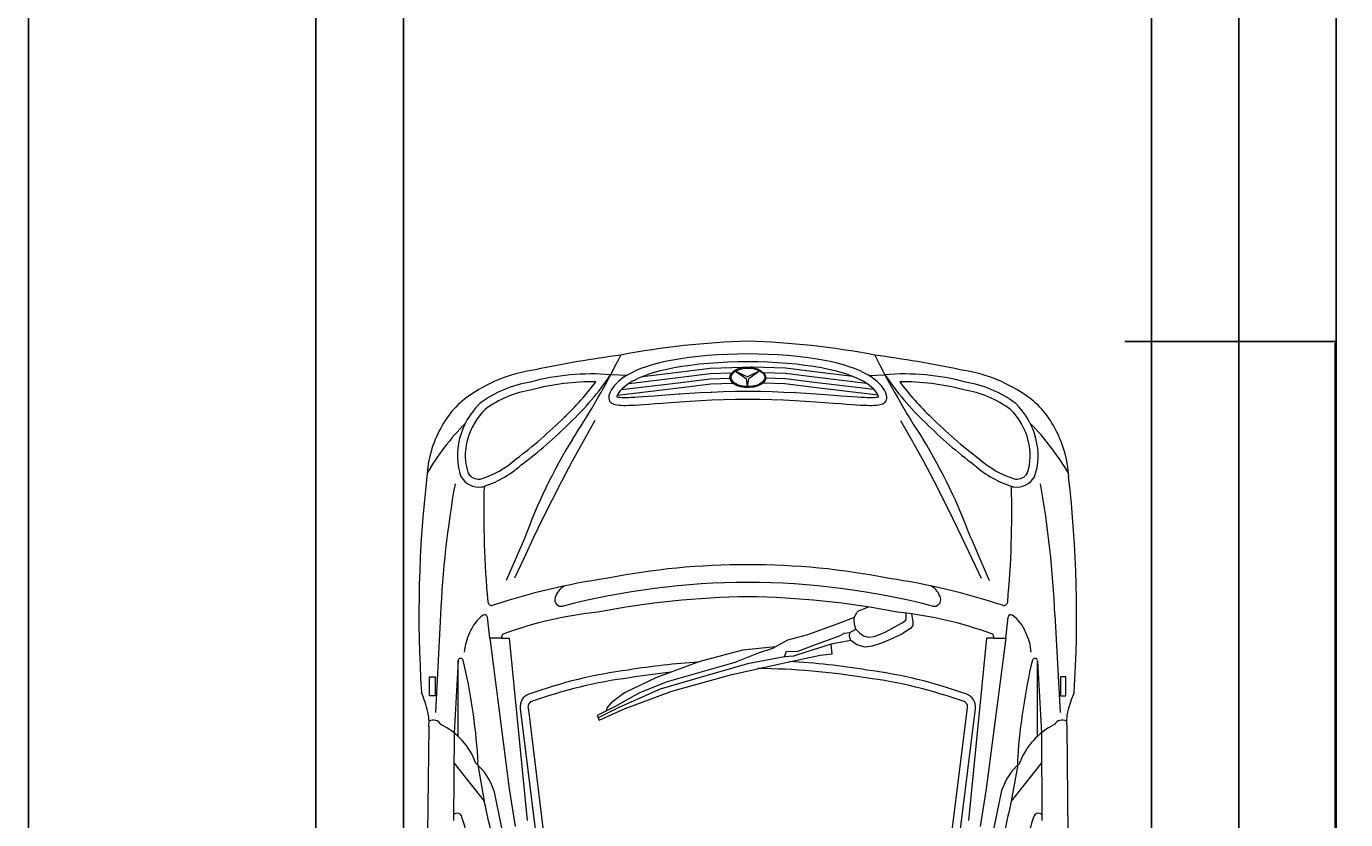
# Model space of a CAD drawing. Units: inches. Extents: x 450 to 1026, y 542 to 1190.
# Tile 3 of 11: x 450 to 586, y 723 to 804. Entities that reach past the tile are written whole.
import ezdxf

# ---------------------------------------------------------------- set-up
doc = ezdxf.new("R2010")
doc.units = ezdxf.units.IN
doc.header["$MEASUREMENT"] = 0
for name, color, linetype, lineweight in [('A-ANNO-DIMS', 2, 'Continuous', 18), ('A-FLOR', 8, 'Continuous', 25), ('C-PROP', 7, 'Continuous', 25), ('C-SITE-VEHC', 8, 'Continuous', 13)]:
    doc.layers.add(name, color=color, linetype=linetype, lineweight=lineweight)
doc.styles.get("Standard").update_dxf_attribs({"font": 'arial.ttf'})
doc.dimstyles.get("Standard").update_dxf_attribs({"dimtxt": 0.18, "dimasz": 0.18, "dimexe": 0.18, "dimexo": 0.0625, "dimgap": 0.09, "dimtad": 0, "dimtih": 1, "dimtoh": 1, "dimdec": 4, "dimzin": 0, "dimdsep": 46, "dimtxsty": 'Standard', "dimcen": 0.09, "dimadec": 0, "dimazin": 0, "dimtfac": 1, "dimtdec": 4, "dimtofl": 0, "dimtmove": 0, "dimatfit": 3, "dimfxl": 1, "dimtolj": 1, "dimtzin": 0, "dimarcsym": 0})

# ---------------------------------------------------------------- blocks, each defined once
blk = doc.blocks.new('A$C27D64469')
for p, q in [((-0.0377, -0.4341), (-0.0629, -0.4354)), ((-0.0122, -0.4333), (-0.0377, -0.4341)), ((0.0136, -0.433), (-0.0122, -0.4333)), ((0.0393, -0.4333), (0.0136, -0.433)), ((0.0649, -0.4341), (0.0393, -0.4333)), ((0.0901, -0.4354), (0.0649, -0.4341)), ((-0.2436, -0.4655), (-0.2571, -0.4703)), ((-0.2289, -0.4609), (-0.2436, -0.4655)), ((-0.2128, -0.4566), (-0.2289, -0.4609)), ((-0.1954, -0.4525), (-0.2128, -0.4566)), ((-0.1764, -0.4487), (-0.1954, -0.4525)), ((-0.156, -0.4453), (-0.1764, -0.4487)), ((-0.153, -0.4651), (-0.1728, -0.4684)), ((-0.1343, -0.4422), (-0.156, -0.4453)), ((-0.1317, -0.4621), (-0.153, -0.4651)), ((-0.1114, -0.4395), (-0.1343, -0.4422)), ((-0.1093, -0.4594), (-0.1317, -0.4621)), ((-0.0875, -0.4373), (-0.1114, -0.4395)), ((-0.0858, -0.4572), (-0.1093, -0.4594)), ((-0.0629, -0.4354), (-0.0875, -0.4373)), ((-0.0616, -0.4554), (-0.0858, -0.4572)), ((-0.0819, -0.4693), (0.0012, -0.4665)), ((-0.0369, -0.4541), (-0.0616, -0.4554)), ((-0.0117, -0.4533), (-0.0369, -0.4541)), ((0.0136, -0.453), (-0.0117, -0.4533)), ((0.0012, -0.4665), (0.0067, -0.4665)), ((0.0389, -0.4533), (0.0136, -0.453)), ((0.0259, -0.4665), (0.0204, -0.4665)), ((0.109, -0.4693), (0.0259, -0.4665)), ((0.064, -0.4541), (0.0389, -0.4533)), ((0.0888, -0.4554), (0.064, -0.4541)), ((0.113, -0.4572), (0.0888, -0.4554)), ((0.1147, -0.4373), (0.0901, -0.4354)), ((0.1364, -0.4594), (0.113, -0.4572)), ((0.1385, -0.4395), (0.1147, -0.4373)), ((0.1588, -0.4621), (0.1364, -0.4594)), ((0.1614, -0.4422), (0.1385, -0.4395)), ((0.1801, -0.4651), (0.1588, -0.4621)), ((0.1832, -0.4453), (0.1614, -0.4422)), ((0.2, -0.4684), (0.1801, -0.4651)), ((0.2036, -0.4487), (0.1832, -0.4453)), ((0.2225, -0.4525), (0.2036, -0.4487)), ((0.24, -0.4566), (0.2225, -0.4525)), ((0.2561, -0.4609), (0.24, -0.4566)), ((0.2708, -0.4655), (0.2561, -0.4609)), ((0.2842, -0.4703), (0.2708, -0.4655)), ((-0.2923, -0.4873), (-0.3337, -0.4857)), ((-0.307, -0.4972), (-0.3138, -0.5028)), ((-0.2991, -0.4915), (-0.307, -0.4972)), ((-0.2902, -0.486), (-0.2991, -0.4915)), ((-0.2803, -0.4806), (-0.2902, -0.486)), ((-0.287, -0.5076), (-0.1557, -0.4919)), ((-0.2693, -0.4753), (-0.2803, -0.4806)), ((-0.2712, -0.4984), (-0.2801, -0.5033)), ((-0.2612, -0.4936), (-0.2712, -0.4984)), ((-0.2571, -0.4703), (-0.2693, -0.4753)), ((-0.2499, -0.489), (-0.2612, -0.4936)), ((-0.253, -0.4902), (-0.1557, -0.4786)), ((-0.2373, -0.4844), (-0.2499, -0.489)), ((-0.2233, -0.4801), (-0.2373, -0.4844)), ((-0.208, -0.476), (-0.2233, -0.4801)), ((-0.1912, -0.4721), (-0.208, -0.476)), ((-0.1728, -0.4684), (-0.1912, -0.4721)), ((-0.1557, -0.4786), (-0.0819, -0.4693)), ((-0.1557, -0.4919), (-0.0819, -0.4825)), ((-0.1557, -0.5051), (-0.0819, -0.4958)), ((-0.0819, -0.4825), (-0.0265, -0.4807)), ((-0.0819, -0.4958), (-0.0315, -0.4941)), ((-0.0174, -0.4766), (0.0132, -0.4908)), ((-0.0174, -0.4766), (0.0101, -0.4961)), ((0.0133, -0.5159), (0.0101, -0.4961)), ((0.0445, -0.4762), (0.0132, -0.4908)), ((0.0133, -0.5159), (0.0162, -0.4961)), ((0.0445, -0.4762), (0.0162, -0.4961)), ((0.109, -0.4825), (0.0537, -0.4807)), ((0.109, -0.4958), (0.0586, -0.4941)), ((0.1828, -0.4786), (0.109, -0.4693)), ((0.1828, -0.4919), (0.109, -0.4825)), ((0.1828, -0.5051), (0.109, -0.4958)), ((0.2801, -0.4902), (0.1828, -0.4786)), ((0.3141, -0.5076), (0.1828, -0.4919)), ((0.2183, -0.4721), (0.2, -0.4684)), ((0.2351, -0.476), (0.2183, -0.4721)), ((0.2505, -0.4801), (0.2351, -0.476)), ((0.2644, -0.4844), (0.2505, -0.4801)), ((0.277, -0.489), (0.2644, -0.4844)), ((0.2883, -0.4936), (0.277, -0.489)), ((0.2964, -0.4753), (0.2842, -0.4703)), ((0.2984, -0.4984), (0.2883, -0.4936)), ((0.3075, -0.4806), (0.2964, -0.4753)), ((0.3073, -0.5033), (0.2984, -0.4984)), ((0.3174, -0.486), (0.3075, -0.4806)), ((0.3262, -0.4915), (0.3174, -0.486)), ((0.3195, -0.4873), (0.3609, -0.4857)), ((0.3341, -0.4972), (0.3262, -0.4915)), ((0.341, -0.5028), (0.3341, -0.4972)), ((-0.3369, -0.5343), (-0.3381, -0.5386)), ((-0.3351, -0.5296), (-0.3369, -0.5343)), ((-0.3324, -0.5247), (-0.3351, -0.5296)), ((-0.329, -0.5195), (-0.3324, -0.5247)), ((-0.3248, -0.514), (-0.329, -0.5195)), ((-0.3198, -0.5085), (-0.3248, -0.514)), ((-0.3138, -0.5028), (-0.3198, -0.5085)), ((-0.3166, -0.5376), (-0.154, -0.5181)), ((-0.3127, -0.5311), (-0.3152, -0.5348)), ((-0.3095, -0.5269), (-0.3127, -0.5311)), ((-0.3055, -0.5225), (-0.3095, -0.5269)), ((-0.306, -0.5231), (-0.1557, -0.5051)), ((-0.3006, -0.5178), (-0.3055, -0.5225)), ((-0.2947, -0.513), (-0.3006, -0.5178)), ((-0.288, -0.5082), (-0.2947, -0.513)), ((-0.2883, -0.5077), (-0.2883, -0.5077)), ((-0.2801, -0.5033), (-0.288, -0.5082)), ((-0.1832, -0.5361), (-0.1598, -0.5344)), ((-0.1597, -0.5344), (-0.1342, -0.5327)), ((-0.154, -0.5181), (-0.0802, -0.5088)), ((-0.1341, -0.5327), (-0.1069, -0.5311)), ((-0.1067, -0.5311), (-0.0781, -0.5297)), ((-0.0802, -0.5088), (-0.0242, -0.5069)), ((-0.0779, -0.5297), (-0.0482, -0.5285)), ((-0.048, -0.5285), (-0.0176, -0.5278)), ((-0.0173, -0.5278), (0.0134, -0.5275)), ((0.0138, -0.5275), (0.0444, -0.5278)), ((0.0448, -0.5278), (0.0751, -0.5285)), ((0.1074, -0.5088), (0.0513, -0.5069)), ((0.0754, -0.5285), (0.105, -0.5297)), ((0.1052, -0.5297), (0.1339, -0.5311)), ((0.1811, -0.5181), (0.1074, -0.5088)), ((0.134, -0.5311), (0.1612, -0.5327)), ((0.1614, -0.5327), (0.1869, -0.5344)), ((0.3438, -0.5376), (0.1811, -0.5181)), ((0.3332, -0.5231), (0.1828, -0.5051)), ((0.187, -0.5344), (0.2103, -0.5361)), ((0.3151, -0.5082), (0.3073, -0.5033)), ((0.3219, -0.513), (0.3151, -0.5082)), ((0.3277, -0.5178), (0.3219, -0.513)), ((0.3326, -0.5225), (0.3277, -0.5178)), ((0.3367, -0.5269), (0.3326, -0.5225)), ((0.3399, -0.5311), (0.3367, -0.5269)), ((0.3423, -0.5348), (0.3399, -0.5311)), ((0.3469, -0.5085), (0.341, -0.5028)), ((0.352, -0.514), (0.3469, -0.5085)), ((0.3562, -0.5195), (0.352, -0.514)), ((0.3596, -0.5247), (0.3562, -0.5195)), ((0.3622, -0.5296), (0.3596, -0.5247)), ((0.3641, -0.5343), (0.3622, -0.5296)), ((0.3653, -0.5386), (0.3641, -0.5343)), ((-0.3381, -0.5386), (-0.3386, -0.5425)), ((-0.3386, -0.5425), (-0.3385, -0.5462)), ((-0.3385, -0.5462), (-0.3378, -0.5495)), ((-0.3378, -0.5495), (-0.3364, -0.5524)), ((-0.3364, -0.5524), (-0.3345, -0.5549)), ((-0.3345, -0.5549), (-0.3321, -0.5571)), ((-0.3321, -0.5571), (-0.3292, -0.5589)), ((-0.3292, -0.5589), (-0.3258, -0.5604)), ((-0.3258, -0.5604), (-0.3219, -0.5615)), ((-0.3219, -0.5615), (-0.3175, -0.5623)), ((-0.318, -0.5407), (-0.3183, -0.5417)), ((-0.3183, -0.5417), (-0.3172, -0.542)), ((-0.3169, -0.5381), (-0.318, -0.5407)), ((-0.3175, -0.5623), (-0.3126, -0.5629)), ((-0.3172, -0.542), (-0.3144, -0.5426)), ((-0.3152, -0.5348), (-0.3169, -0.5381)), ((-0.3144, -0.5426), (-0.3108, -0.543)), ((-0.3126, -0.5629), (-0.3072, -0.5633)), ((-0.3108, -0.543), (-0.3063, -0.5433)), ((-0.3072, -0.5633), (-0.3014, -0.5634)), ((-0.3063, -0.5433), (-0.3012, -0.5434)), ((-0.3014, -0.5634), (-0.2951, -0.5634)), ((-0.3012, -0.5434), (-0.2953, -0.5434)), ((-0.2953, -0.5434), (-0.2888, -0.5433)), ((-0.2951, -0.5634), (-0.2882, -0.5633)), ((-0.2888, -0.5433), (-0.2815, -0.543)), ((-0.2882, -0.5633), (-0.2806, -0.563)), ((-0.2815, -0.543), (-0.2731, -0.5425)), ((-0.2806, -0.563), (-0.272, -0.5625)), ((-0.2731, -0.5425), (-0.2632, -0.5419)), ((-0.272, -0.5625), (-0.2619, -0.5619)), ((-0.2632, -0.5419), (-0.2517, -0.5411)), ((-0.2619, -0.5619), (-0.2503, -0.5611)), ((-0.2517, -0.5411), (-0.2382, -0.5402)), ((-0.2503, -0.5611), (-0.2367, -0.5601)), ((-0.2382, -0.5402), (-0.2225, -0.539)), ((-0.2367, -0.5601), (-0.221, -0.559)), ((-0.2225, -0.539), (-0.2042, -0.5376)), ((-0.221, -0.559), (-0.2027, -0.5576)), ((-0.2042, -0.5376), (-0.1833, -0.5361)), ((-0.2027, -0.5576), (-0.1818, -0.556)), ((-0.1818, -0.556), (-0.1584, -0.5544)), ((-0.1584, -0.5544), (-0.1329, -0.5527)), ((-0.1329, -0.5527), (-0.1057, -0.5511)), ((-0.1057, -0.5511), (-0.0771, -0.5496)), ((-0.0771, -0.5496), (-0.0475, -0.5485)), ((-0.0475, -0.5485), (-0.0171, -0.5478)), ((-0.0171, -0.5478), (0.0136, -0.5475)), ((0.0136, -0.5475), (0.0443, -0.5478)), ((0.0443, -0.5478), (0.0746, -0.5485)), ((0.0746, -0.5485), (0.1043, -0.5496)), ((0.1043, -0.5496), (0.1329, -0.5511)), ((0.1329, -0.5511), (0.1601, -0.5527)), ((0.1601, -0.5527), (0.1855, -0.5544)), ((0.1855, -0.5544), (0.2089, -0.556)), ((0.2089, -0.556), (0.2299, -0.5576)), ((0.2104, -0.5361), (0.2314, -0.5376)), ((0.2299, -0.5576), (0.2481, -0.559)), ((0.2314, -0.5376), (0.2496, -0.539)), ((0.2481, -0.559), (0.2639, -0.5601)), ((0.2496, -0.539), (0.2653, -0.5402)), ((0.2639, -0.5601), (0.2775, -0.5611)), ((0.2653, -0.5402), (0.2788, -0.5411)), ((0.2775, -0.5611), (0.2891, -0.5619)), ((0.2788, -0.5411), (0.2904, -0.5419)), ((0.2891, -0.5619), (0.2991, -0.5625)), ((0.2904, -0.5419), (0.3002, -0.5425)), ((0.2991, -0.5625), (0.3078, -0.563)), ((0.3002, -0.5425), (0.3087, -0.543)), ((0.3078, -0.563), (0.3154, -0.5633)), ((0.3087, -0.543), (0.316, -0.5433)), ((0.3154, -0.5633), (0.3222, -0.5634)), ((0.316, -0.5433), (0.3225, -0.5434)), ((0.3222, -0.5634), (0.3285, -0.5634)), ((0.3225, -0.5434), (0.3283, -0.5434)), ((0.3283, -0.5434), (0.3335, -0.5433)), ((0.3285, -0.5634), (0.3344, -0.5633)), ((0.3335, -0.5433), (0.3379, -0.543)), ((0.3344, -0.5633), (0.3398, -0.5629)), ((0.3379, -0.543), (0.3416, -0.5426)), ((0.3398, -0.5629), (0.3446, -0.5623)), ((0.3416, -0.5426), (0.3444, -0.542)), ((0.3441, -0.5381), (0.3423, -0.5348)), ((0.3451, -0.5407), (0.3441, -0.5381)), ((0.3444, -0.542), (0.3454, -0.5417)), ((0.3446, -0.5623), (0.349, -0.5615)), ((0.3454, -0.5417), (0.3451, -0.5407)), ((0.349, -0.5615), (0.3529, -0.5604)), ((0.3529, -0.5604), (0.3563, -0.5589)), ((0.3563, -0.5589), (0.3593, -0.5571)), ((0.3593, -0.5571), (0.3617, -0.5549)), ((0.3617, -0.5549), (0.3636, -0.5524)), ((0.3636, -0.5524), (0.3649, -0.5495)), ((0.3649, -0.5495), (0.3656, -0.5462)), ((0.3658, -0.5425), (0.3653, -0.5386)), ((0.3656, -0.5462), (0.3658, -0.5425)), ((-0.3736, -0.602), (-0.4036, -0.6546)), ((0.4008, -0.602), (0.4307, -0.6546)), ((-0.4036, -0.6546), (-0.4313, -0.7051)), ((0.4307, -0.6546), (0.4585, -0.7051)), ((-0.4313, -0.7051), (-0.4574, -0.7542)), ((0.4585, -0.7051), (0.4846, -0.7542)), ((-0.4574, -0.7542), (-0.4822, -0.8025)), ((0.4846, -0.7542), (0.5094, -0.8025)), ((-0.4822, -0.8025), (-0.5062, -0.8507)), ((0.5094, -0.8025), (0.5333, -0.8507)), ((-0.5062, -0.8507), (-0.5297, -0.8995)), ((0.5333, -0.8507), (0.5568, -0.8995)), ((-0.552, -0.901), (-0.5982, -1.0071)), ((-0.5297, -0.8995), (-0.5532, -0.9495)), ((0.5568, -0.8995), (0.5804, -0.9495)), ((0.5791, -0.901), (0.6253, -1.0071)), ((-0.5532, -0.9495), (-0.5772, -1.0014)), ((0.5804, -0.9495), (0.6044, -1.0014)), ((-0.7646, -1.0944), (-0.7774, -1.3418)), ((-0.6398, -1.1535), (-0.646, -1.0999)), ((0.2832, -1.1011), (0.2417, -1.1168)), ((0.283, -1.1095), (0.2832, -1.1011)), ((0.2832, -1.1011), (0.2905, -1.0871)), ((0.2925, -1.0852), (0.3197, -1.0743)), ((0.4151, -1.1035), (0.4148, -1.0897)), ((0.4283, -1.0915), (0.4315, -1.1115)), ((0.6669, -1.1535), (0.6731, -1.0999)), ((0.7917, -1.0944), (0.8046, -1.3418)), ((0.2417, -1.1168), (0.1646, -1.1448)), ((0.2722, -1.1385), (0.2873, -1.1305)), ((0.2848, -1.1224), (0.283, -1.1095)), ((0.2873, -1.1305), (0.2848, -1.1224)), ((0.2873, -1.1305), (0.2969, -1.1395)), ((0.3634, -1.137), (0.3841, -1.1257)), ((0.3841, -1.1257), (0.4048, -1.1143)), ((0.4254, -1.1287), (0.4022, -1.1436)), ((0.4048, -1.1143), (0.4131, -1.1088)), ((0.4131, -1.1088), (0.4151, -1.106)), ((0.4151, -1.106), (0.4151, -1.1035)), ((0.4315, -1.1216), (0.4254, -1.1287)), ((0.4315, -1.1115), (0.4315, -1.1216)), ((-0.6398, -1.1535), (-0.5904, -1.5351)), ((-0.61, -1.1535), (-0.6398, -1.1535)), ((-0.61, -1.1535), (-0.5908, -1.1535)), ((-0.5908, -1.1535), (-0.5454, -1.6151)), ((0.1143, -1.158), (0.0761, -1.1797)), ((0.1646, -1.1448), (0.1143, -1.158)), ((0.1383, -1.1871), (0.188, -1.1683)), ((0.2252, -1.1688), (0.1635, -1.1877)), ((0.188, -1.1683), (0.2457, -1.1477)), ((0.2271, -1.1931), (0.2246, -1.169)), ((0.2744, -1.1592), (0.2252, -1.1688)), ((0.2457, -1.1477), (0.2589, -1.1408)), ((0.2589, -1.1408), (0.2722, -1.1385)), ((0.2711, -1.1491), (0.2722, -1.1385)), ((0.2744, -1.1592), (0.2711, -1.1491)), ((0.2895, -1.1703), (0.2744, -1.1592)), ((0.2969, -1.1395), (0.3069, -1.1474)), ((0.3069, -1.1474), (0.3193, -1.1504)), ((0.3193, -1.1504), (0.3339, -1.1491)), ((0.3526, -1.1658), (0.3289, -1.1738)), ((0.3339, -1.1491), (0.3475, -1.1443)), ((0.3475, -1.1443), (0.3634, -1.137)), ((0.3745, -1.1567), (0.3526, -1.1658)), ((0.4022, -1.1436), (0.3745, -1.1567)), ((0.618, -1.1535), (0.5726, -1.6151)), ((0.6669, -1.1535), (0.6175, -1.5351)), ((0.6371, -1.1535), (0.618, -1.1535)), ((0.6371, -1.1535), (0.6669, -1.1535)), ((0, -1.1841), (-0.1108, -1.2136)), ((0.0401, -1.1917), (-0.0188, -1.2151)), ((0.0839, -1.1753), (0, -1.1841)), ((0.1069, -1.2008), (0.013, -1.2184)), ((0.0761, -1.1797), (0.0401, -1.1917)), ((0.1062, -1.2154), (0.1972, -1.1964)), ((0.1069, -1.2008), (0.112, -1.1865)), ((0.1298, -1.1986), (0.1069, -1.2008)), ((0.112, -1.1865), (0.1383, -1.1871)), ((0.1635, -1.1877), (0.1298, -1.1986)), ((0.1972, -1.1964), (0.2271, -1.1931)), ((0.3107, -1.1759), (0.2895, -1.1703)), ((0.3289, -1.1738), (0.3107, -1.1759)), ((-0.7203, -1.2103), (-0.7302, -1.3933)), ((-0.7203, -1.4019), (-0.7203, -1.2103)), ((-0.1108, -1.2136), (-0.2189, -1.2538)), ((-0.0188, -1.2151), (-0.1903, -1.264)), ((0.013, -1.2184), (-0.1069, -1.2532)), ((-0.0266, -1.2451), (0.1062, -1.2154)), ((0.7474, -1.4019), (0.7474, -1.2103)), ((0.7474, -1.2103), (0.7573, -1.3933)), ((-0.7922, -1.2996), (-0.7922, -1.251)), ((-0.7922, -1.251), (-0.7785, -1.251)), ((-0.7785, -1.251), (-0.7785, -1.2996)), ((-0.2189, -1.2538), (-0.2983, -1.2922)), ((-0.1903, -1.264), (-0.2605, -1.2919)), ((-0.1069, -1.2532), (-0.2084, -1.2823)), ((-0.1789, -1.2879), (-0.0266, -1.2451)), ((0.8056, -1.251), (0.8056, -1.2996)), ((0.8193, -1.251), (0.8056, -1.251)), ((0.8193, -1.2996), (0.8193, -1.251)), ((-0.7785, -1.2996), (-0.7922, -1.2996)), ((-0.2983, -1.2922), (-0.3323, -1.3172)), ((-0.2605, -1.2919), (-0.3222, -1.3262)), ((-0.2084, -1.2823), (-0.3128, -1.3287)), ((-0.2968, -1.3312), (-0.1789, -1.2879)), ((0.8056, -1.2996), (0.8193, -1.2996)), ((-0.563, -1.3311), (-0.5244, -1.6438)), ((-0.5431, -1.3287), (-0.5046, -1.6408)), ((-0.3222, -1.3262), (-0.3675, -1.3491)), ((-0.3128, -1.3287), (-0.3653, -1.355)), ((-0.363, -1.3611), (-0.2968, -1.3312)), ((-0.343, -1.3297), (-0.345, -1.3377)), ((-0.3323, -1.3172), (-0.343, -1.3297)), ((0.5317, -1.6408), (0.5703, -1.3287)), ((0.5515, -1.6438), (0.5901, -1.3311)), ((-0.3675, -1.3491), (-0.363, -1.3611)), ((-0.7946, -1.3764), (-0.7975, -1.6481)), ((-0.7302, -1.3933), (-0.7314, -1.6155)), ((0.7573, -1.3933), (0.7586, -1.6155)), ((0.8217, -1.3764), (0.8246, -1.6481)), ((-0.7306, -1.4695), (-0.6539, -1.5666)), ((0.7578, -1.4695), (0.681, -1.5666)), ((-0.6702, -1.4746), (-0.6539, -1.5666)), ((0.6973, -1.4746), (0.681, -1.5666)), ((-0.5904, -1.5351), (-0.5754, -1.6301)), ((0.6175, -1.5351), (0.6026, -1.6301)), ((-0.6294, -1.5396), (-0.5492, -1.9272)), ((0.6565, -1.5396), (0.5764, -1.9272))]:
    blk.add_line(p, q)
for centre, radius, start, end in [((0.0637, -2.359), 1.9586, 91.468, 100.9476), ((-0.0366, -2.359), 1.9586, 79.0524, 88.532), ((0.1265, -3.625), 3.2185, 97.7633, 101.6634), ((-2.1519, 0.4791), 2.0583, 326.7435, 333.6014), ((-0.0994, -3.625), 3.2185, 78.3366, 82.2367), ((2.179, 0.4791), 2.0583, 206.3986, 213.2565), ((-0.471, -0.8549), 0.3855, 97.9189, 123.9683), ((-0.3813, -1.088), 0.6042, 85.4848, 104.9936), ((-0.9467, -0.0711), 0.74, 313.509, 325.9238), ((0.4084, -1.088), 0.6042, 75.0064, 94.5152), ((0.9738, -0.0711), 0.74, 214.0762, 226.491), ((0.4981, -0.8549), 0.3855, 56.0317, 82.0811), ((-0.4915, -0.79), 0.2893, 99.1695, 126.8677), ((-0.4915, -0.79), 0.2693, 98.9551, 126.5901), ((-0.3813, -1.088), 0.5842, 89.0187, 105.0943), ((-0.9467, -0.0711), 0.72, 313.4908, 323.0478), ((-0.1584, -0.5544), 0.02, 93.7902, 94.094), ((-0.1329, -0.5527), 0.02, 93.3698, 93.7902), ((-0.1057, -0.5511), 0.02, 92.8387, 93.3698), ((-0.0771, -0.5496), 0.02, 92.1933, 92.8387), ((-0.0475, -0.5485), 0.02, 91.423, 92.1933), ((-0.0171, -0.5478), 0.02, 90.5101, 91.423), ((0.0136, -0.5475), 0.02, 89.4899, 90.5101), ((0.0443, -0.5478), 0.02, 88.577, 89.4899), ((0.0746, -0.5485), 0.02, 87.8067, 88.577), ((0.1043, -0.5496), 0.02, 87.1613, 87.8067), ((0.1329, -0.5511), 0.02, 86.6302, 87.1613), ((0.1601, -0.5527), 0.02, 86.2098, 86.6302), ((0.1855, -0.5544), 0.02, 85.906, 86.2098), ((0.4084, -1.088), 0.5842, 74.9057, 90.9813), ((0.9738, -0.0711), 0.72, 216.9522, 226.5092), ((0.5186, -0.79), 0.2693, 53.4099, 81.0449), ((0.5186, -0.79), 0.2893, 53.1323, 80.8305), ((-0.5677, -0.7201), 0.2198, 122.6776, 153.2639), ((-0.5339, -0.6931), 0.1879, 134.257, 165.9979), ((-0.2027, -0.5576), 0.02, 94.2621, 94.2814), ((-0.1818, -0.556), 0.02, 94.094, 94.2621), ((0.2089, -0.556), 0.02, 85.7379, 85.906), ((0.2299, -0.5576), 0.02, 85.7186, 85.7379), ((0.5611, -0.6931), 0.1879, 14.0021, 45.743), ((0.5949, -0.7201), 0.2198, 26.7361, 57.3224), ((-0.5339, -0.6931), 0.1679, 134.6933, 166.0746), ((-1.2622, 0.2224), 1.1505, 306.8088, 314.8317), ((1.2894, 0.2224), 1.1505, 225.1683, 233.1912), ((0.5611, -0.6931), 0.1679, 13.9254, 45.3067), ((-0.5196, -0.7579), 0.2801, 150.7841, 177.1611), ((-0.2571, -1.0501), 0.6264, 135.2689, 149.8576), ((-1.2622, 0.2224), 1.1705, 306.853, 314.8203), ((1.2894, 0.2224), 1.1705, 225.1797, 233.147), ((0.2842, -1.0501), 0.6264, 30.1424, 44.7311), ((0.5467, -0.7579), 0.2801, 2.8389, 29.2159), ((-0.5599, -0.6904), 0.1621, 164.7178, 199.3716), ((-0.5599, -0.6904), 0.1421, 164.6281, 198.5509), ((0.7633, -1.3808), 1.4001, 148.5187, 159.9579), ((-0.7362, -1.3808), 1.4001, 20.0421, 31.4813), ((0.587, -0.6904), 0.1421, 341.4491, 15.3719), ((0.587, -0.6904), 0.1621, 340.6284, 15.2822), ((-0.7354, -0.5187), 0.2425, 286.9921, 312.0664), ((0.7625, -0.5187), 0.2425, 227.9336, 253.0079), ((-0.7354, -0.5187), 0.2625, 286.5483, 311.8628), ((0.7625, -0.5187), 0.2625, 228.1372, 253.4517), ((2.2292, -1.0935), 3.0486, 173.4174, 183.7163), ((1.7769, -1.2069), 2.544, 169.9235, 177.4667), ((-0.6669, -0.7176), 0.053, 210.0698, 276.7845), ((-0.6669, -0.7176), 0.033, 213.0457, 274.1097), ((1.7667, -0.8364), 2.422, 178.3888, 185.3284), ((-1.7396, -0.8364), 2.422, 354.6716, 1.6112), ((0.694, -0.7176), 0.053, 263.2155, 329.9302), ((0.694, -0.7176), 0.033, 265.8903, 326.9543), ((-1.7498, -1.2069), 2.544, 2.5333, 10.0765), ((-2.2021, -1.0935), 3.0486, 356.2837, 6.5826), ((0.0046, -2.7444), 1.777, 89.7096, 101.339), ((0.0226, -2.7444), 1.777, 78.661, 90.2904), ((-0.1068, -2.6471), 1.6622, 98.2339, 108.4059), ((0.1339, -2.6471), 1.6622, 71.5941, 81.7661), ((-0.4223, -1.0677), 0.055, 122.1615, 161.7809), ((0.0163, -2.8903), 1.8782, 90.0843, 104.512), ((0.0108, -2.8903), 1.8782, 75.488, 89.9157), ((0.4494, -1.0677), 0.055, 18.2191, 57.8385), ((-0.6348, -1.0604), 0.0101, 185.3284, 288.4059), ((-0.4585, -1.0557), 0.0168, 161.7809, 284.512), ((0.0393, -3.1787), 2.1304, 90.6925, 100.9626), ((-0.0122, -3.1787), 2.1304, 79.0374, 89.3075), ((0.4857, -1.0557), 0.0168, 255.488, 18.2191), ((0.6619, -1.0604), 0.0101, 251.5941, 354.6716), ((-0.6033, -1.1719), 0.0933, 124.7249, 159.8848), ((-0.6527, -1.1007), 0.00673, 6.5512, 124.7249), ((-0.2611, -2.0848), 1.0031, 95.9948, 110.0315), ((0.294, -1.0889), 0.004, 111.8862, 152.6845), ((0.2882, -2.0848), 1.0031, 69.9685, 84.0052), ((0.6798, -1.1007), 0.00673, 55.2751, 173.4488), ((0.6305, -1.1719), 0.0933, 20.1152, 55.2751), ((-0.5552, -1.2042), 0.1503, 154.6022, 174.0364), ((-0.5998, -1.1515), 0.0104, 118.0528, 191.1071), ((0.6269, -1.1515), 0.0104, 348.8929, 61.9472), ((0.5823, -1.2042), 0.1503, 5.9636, 25.3978), ((-0.7137, -1.2111), 0.00665, 15.5251, 172.9634), ((-2.218, -1.5637), 1.5518, 4.0302, 13.202), ((-0.1308, -2.4351), 1.2114, 97.4669, 109.7935), ((0.0017, -2.9892), 1.779, 93.6503, 99.3781), ((0.0254, -2.9892), 1.759, 80.6111, 89.5421), ((0.0254, -2.9892), 1.779, 80.6219, 86.9829), ((0.1579, -2.4351), 1.2114, 70.2065, 82.5331), ((2.2452, -1.5637), 1.5518, 166.798, 175.9698), ((0.7408, -1.2111), 0.00665, 7.0366, 164.4749), ((-0.1308, -2.4351), 1.1914, 97.4508, 109.7935), ((0.0017, -2.9892), 1.759, 95.9707, 99.3889), ((0.1579, -2.4351), 1.1914, 70.2065, 82.5492), ((-1.1013, -1.4136), 0.3132, 13.4845, 23.0084), ((-0.5296, -1.327), 0.0337, 109.7935, 187.0357), ((0.5567, -1.327), 0.0337, 352.9643, 70.2065), ((1.1284, -1.4136), 0.3132, 156.9916, 166.5155), ((-0.5296, -1.327), 0.0137, 109.7935, 187.0357), ((0.5567, -1.327), 0.0137, 352.9643, 70.2065), ((-0.8898, -1.3641), 0.096, 352.6385, 14.2173), ((-0.7831, -1.3832), 0.0225, 29.7837, 118.4161), ((0.8102, -1.3832), 0.0225, 61.5839, 150.2163), ((0.9169, -1.3641), 0.096, 165.7827, 187.3615), ((-0.8418, -1.5314), 0.1776, 20.2536, 63.8557), ((0.8689, -1.5314), 0.1776, 116.1443, 159.7464), ((-0.7826, -1.5905), 0.1615, 18.3646, 48.2784), ((-0.771, -1.4642), 0.1013, 354.1028, 5.3715), ((0.8098, -1.5905), 0.1615, 131.7216, 161.6354), ((0.7981, -1.4642), 0.1013, 174.6285, 185.8972), ((-10.825, -3.8887), 10.4328, 11.75206, 12.86028), ((10.8521, -3.8887), 10.4328, 167.13972, 168.24794), ((-0.7227, -1.6094), 0.0124, 11.3416, 134.5987), ((0.7498, -1.6094), 0.0124, 45.4013, 168.6584), ((-0.9441, -1.6953), 0.2497, 351.6082, 20.7105), ((0.9712, -1.6953), 0.2497, 159.2895, 188.3918)]:
    blk.add_arc(centre, radius, start, end)
blk.add_ellipse((0.014, -0.4925), major_axis=(-0.0426, 0), ratio=0.550187)
blk.add_open_spline([(-0.0315, -0.4925), (-0.0315, -0.5012), (-0.0242, -0.5089), (0.0098, -0.5237), (0.0496, -0.5174), (0.0659, -0.4821), (0.0357, -0.4635), (-0.0133, -0.4686), (-0.0315, -0.4789), (-0.0315, -0.4925)], degree=3, knots=[0, 0, 0, 0, 0.903923, 0.903923, 2.878844, 2.878844, 4.872977, 4.872977, 6.283185, 6.283185, 6.283185, 6.283185])
blk = doc.blocks.new('*D43')
at = {"layer": 'A-ANNO-DIMS', "color": 0, "lineweight": -2, "transparency": 16777216}
for p, q in [((562.89, 771.86), (584.74, 771.86)), ((584.56, 771.68), (584.56, 699.59)), ((584.56, 627.13), (584.56, 699.22)), ((562.89, 626.95), (584.74, 626.95))]:
    blk.add_line(p, q, dxfattribs=at)
at = {"layer": 'A-ANNO-DIMS', "color": 0, "transparency": 16777216}
for points in [[(584.53, 771.68), (584.59, 771.68), (584.56, 771.86)], [(584.53, 627.13), (584.59, 627.13), (584.56, 626.95)]]:
    blk.add_solid(points, dxfattribs=at)
at = {"layer": 'Defpoints', "color": 0, "transparency": 16777216}
for p in [(562.83, 771.86), (584.56, 771.86), (562.83, 626.95)]:
    blk.add_point(p, dxfattribs=at)
at = {"layer": 'A-ANNO-DIMS', "color": 0, "transparency": 16777216, "insert": (584.56, 699.41), "char_height": 0.18, "attachment_point": 5}
blk.add_mtext('\\A1;VEHICLE 145', dxfattribs=at)
blk = doc.blocks.new('*D53')
at = {"layer": 'A-ANNO-DIMS', "color": 0, "lineweight": -2, "transparency": 16777216}
for p, q in [((479.59, 817.94), (449.87, 817.94)), ((450.05, 817.76), (450.05, 706.62)), ((450.05, 595.12), (450.05, 706.26)), ((797.59, 594.94), (449.87, 594.94))]:
    blk.add_line(p, q, dxfattribs=at)
at = {"layer": 'A-ANNO-DIMS', "color": 0, "transparency": 16777216}
for points in [[(450.02, 817.76), (450.08, 817.76), (450.05, 817.94)], [(450.02, 595.12), (450.08, 595.12), (450.05, 594.94)]]:
    blk.add_solid(points, dxfattribs=at)
at = {"layer": 'Defpoints', "color": 0, "transparency": 16777216}
for p in [(479.65, 817.94), (450.05, 594.94), (797.65, 594.94)]:
    blk.add_point(p, dxfattribs=at)
at = {"layer": 'A-ANNO-DIMS', "color": 0, "transparency": 16777216, "insert": (450.05, 706.44), "char_height": 0.18, "attachment_point": 5}
blk.add_mtext('\\A1;223', dxfattribs=at)
blk = doc.blocks.new('*D56')
at = {"layer": 'A-ANNO-DIMS', "color": 0, "lineweight": -2, "transparency": 16777216}
for p, q in [((488.65, 1150.88), (488.65, 542.16)), ((584.65, 1150.88), (584.65, 542.16)), ((488.83, 542.34), (536.43, 542.34)), ((584.47, 542.34), (536.87, 542.34))]:
    blk.add_line(p, q, dxfattribs=at)
at = {"layer": 'A-ANNO-DIMS', "color": 0, "transparency": 16777216}
for points in [[(488.83, 542.37), (488.83, 542.31), (488.65, 542.34)], [(584.47, 542.37), (584.47, 542.31), (584.65, 542.34)]]:
    blk.add_solid(points, dxfattribs=at)
at = {"layer": 'Defpoints', "color": 0, "transparency": 16777216}
for p in [(488.65, 1150.94), (584.65, 1150.94), (584.65, 542.34)]:
    blk.add_point(p, dxfattribs=at)
at = {"layer": 'A-ANNO-DIMS', "color": 0, "transparency": 16777216, "insert": (536.65, 542.34), "char_height": 0.18, "attachment_point": 5}
blk.add_mtext('\\A1;96', dxfattribs=at)
blk = doc.blocks.new('*D70')
at = {"layer": 'A-ANNO-DIMS', "color": 0, "lineweight": -2, "transparency": 16777216}
for p, q in [((565.65, 713.01), (565.65, 1189.72)), ((565.83, 1189.54), (580.43, 1189.54)), ((595.47, 1189.54), (580.87, 1189.54)), ((595.65, 713.01), (595.65, 1189.72))]:
    blk.add_line(p, q, dxfattribs=at)
at = {"layer": 'A-ANNO-DIMS', "color": 0, "transparency": 16777216}
for points in [[(565.83, 1189.57), (565.83, 1189.51), (565.65, 1189.54)], [(595.47, 1189.57), (595.47, 1189.51), (595.65, 1189.54)]]:
    blk.add_solid(points, dxfattribs=at)
at = {"layer": 'Defpoints', "color": 0, "transparency": 16777216}
for p in [(595.65, 1189.54), (565.65, 712.94), (595.65, 712.94)]:
    blk.add_point(p, dxfattribs=at)
at = {"layer": 'A-ANNO-DIMS', "color": 0, "transparency": 16777216, "insert": (580.65, 1189.54), "char_height": 0.18, "attachment_point": 5}
blk.add_mtext('\\A1;30', dxfattribs=at)

msp = doc.modelspace()

# ---------------------------------------------------------------- linework, layer by layer
at = {"layer": 'A-FLOR'}
for points in [[(565.6513, 826.9426), (565.6513, 712.9426, 0.41421356), (637.6513, 640.9426), (797.6513, 640.9426)], [(574.6513, 826.9426), (574.6513, 721.9426, 0.41421356), (646.6513, 649.9426), (797.6513, 649.9426)]]:
    msp.add_lwpolyline(points, format="xyb", dxfattribs=at)
at = {"layer": 'C-PROP'}
msp.add_line((479.6513, 1159.9426), (479.6513, 571.9426), dxfattribs=at)

# ---------------------------------------------------------------- block references
at = {"layer": 'C-SITE-VEHC', "xscale": 40.63350989877505, "yscale": 40.63350989877505, "zscale": 40.63350989877505}
msp.add_blockref('A$C27D64469', (523.5448, 788.1608), dxfattribs=at)

# ---------------------------------------------------------------- dimensions: what is measured, and where the dimension line sits
at = {"layer": 'A-ANNO-DIMS'}
for base, p1, p2, picture, middle in [((595.6513, 1189.5426), (565.6513, 712.9426), (595.6513, 712.9426), '*D70', (580.6513, 1189.5426)), ((584.6513, 542.3426), (488.6513, 1150.9426), (584.6513, 1150.9426), '*D56', (536.6513, 542.3426))]:
    dim = msp.add_linear_dim(base=base, p1=p1, p2=p2, dimstyle='Standard', override={"dimdec": 0, "dimlfac": 1, "dimrnd": 0, "dimzin": 0, "dimdsep": 46, "dimlunit": 2}, dxfattribs=at)
    dim.commit()
    dim.dimension.update_dxf_attribs({"geometry": picture, "text_midpoint": middle})
dim = msp.add_linear_dim(base=(450.0513, 594.9426), p1=(479.6513, 817.9426), p2=(797.6513, 594.9426), angle=90, dimstyle='Standard', override={"dimdec": 0, "dimlfac": 1, "dimrnd": 0, "dimzin": 0, "dimdsep": 46, "dimlunit": 2}, dxfattribs=at)
dim.commit()
dim.dimension.update_dxf_attribs({"geometry": '*D53', "text_midpoint": (450.0513, 706.4426)})
dim = msp.add_linear_dim(base=(584.563, 771.8648), p1=(562.8259, 626.9507), p2=(562.8259, 771.8648), angle=90, text='VEHICLE <>', dimstyle='Standard', override={"dimdec": 0, "dimlfac": 1, "dimrnd": 0, "dimzin": 0, "dimdsep": 46, "dimlunit": 2}, dxfattribs=at)
dim.commit()
dim.dimension.update_dxf_attribs({"geometry": '*D43', "text_midpoint": (584.563, 699.4077)})

doc.saveas('drawing.dxf')
